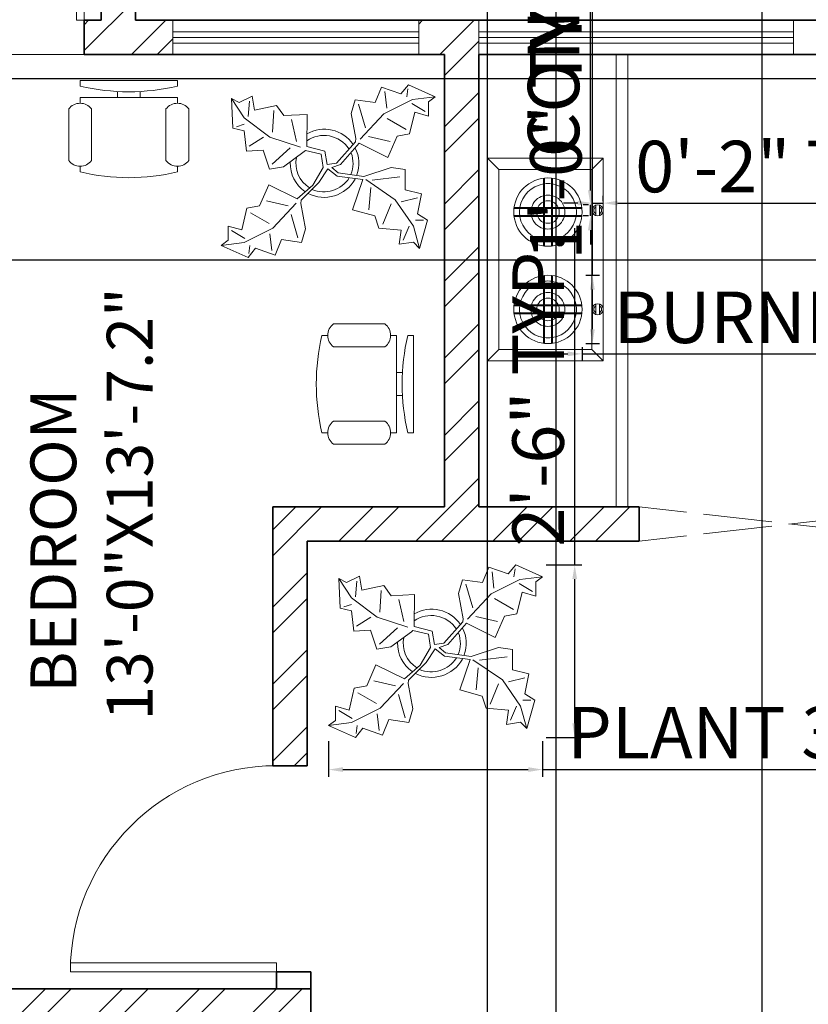
# Model space of a CAD drawing. Units: inches. Extents: x 744 to 1448, y 5126 to 6077.
# Tile 6 of 10: x 895 to 1033, y 5585 to 5757. Entities that reach past the tile are written whole.
import ezdxf

# ---------------------------------------------------------------- set-up
doc = ezdxf.new("R2010")
doc.units = ezdxf.units.IN
doc.linetypes.add('ACAD_ISO02W100', pattern=[15, 12, -3])
for name, color, linetype, lineweight in [('A-ANNO-DIMS', 2, 'Continuous', 18), ('A-AREA-IDEN', 7, 'Continuous', 18), ('A-DOOR', 4, 'Continuous', 18), ('A-EQPM', 9, 'Continuous', 18), ('A-FLOR-CASE', 8, 'Continuous', 18), ('A-FURN', 8, 'Continuous', 18), ('A-WALL', 7, 'Continuous', 35), ('A-WALL-PATT', 252, 'Continuous', 13), ('L-PLNT', 3, 'Continuous', 13)]:
    doc.layers.add(name, color=color, linetype=linetype, lineweight=lineweight)
doc.layers.add('A-GLAZ', color=244, linetype='Continuous', lineweight=18, true_color=0x991b1e)
doc.layers.add('A-WALL-OVHD', color=244, linetype='ACAD_ISO02W100', lineweight=13, true_color=0x991b1e)
doc.styles.get("Standard").update_dxf_attribs({"font": 'arial.ttf'})
doc.dimstyles.new('ISO-25', dxfattribs={"dimtxt": 9, "dimasz": 2.5, "dimexe": 1.25, "dimexo": 0.625, "dimtad": 1, "dimlunit": 3, "dimtxsty": 'Standard', "dimcen": 2.5, "dimadec": 0, "dimazin": 0, "dimtfac": 1, "dimtmove": 0, "dimatfit": 3, "dimfxl": 1, "dimarcsym": 0})

# ---------------------------------------------------------------- blocks, each defined once
blk = doc.blocks.new('*U2')
for p, q in [((0, 0), (0, -6)), ((40, 0), (40, -6))]:
    blk.add_line(p, q)
blk.add_lwpolyline([(0, 0), (0, 40), (1.75, 40), (1.75, 0)], close=True)
blk.add_arc((0, 0), 40, 0, 90)
blk = doc.blocks.new('*U4')
for p, q in [((0, 0), (0, 6)), ((40, 0), (40, 6))]:
    blk.add_line(p, q)
blk.add_lwpolyline([(0, 0), (0, -40), (1.75, -40), (1.75, 0)], close=True)
blk.add_arc((0, 0), 40, 270, 0)
blk = doc.blocks.new('Plant - Rubber or Philodendron')
for p, q in [((13.3837, 12.301), (14.68, 13.9039)), ((14.68, 13.9039), (19.3848, 11.8146)), ((8.8871, 10.7908), (9.9809, 13.4933)), ((9.9809, 13.4933), (13.3837, 12.301)), ((10.5828, 12.6946), (10.8893, 9.7953)), ((14.5816, 13.2037), (14.3848, 11.8033)), ((-16.2005, 11.4774), (-13.9899, 8.1064)), ((-16.2005, 11.4774), (-14.8639, 10.7964)), ((-16.0159, 6.3329), (-16.2005, 11.4774)), ((-14.8639, 10.7964), (-12.6195, 11.8975)), ((-13.3174, 8.325), (-13.0735, 11.0065)), ((-12.6195, 11.8975), (-12.1909, 9.4345)), ((4.6914, 8.8812), (5.3859, 11.2828)), ((5.3859, 11.2828), (8.8871, 10.7908)), ((5.9878, 10.4842), (7.1971, 6.3869)), ((15.3859, 11.3055), (10.3916, 8.7942)), ((15.2875, 10.6053), (17.5907, 9.2105)), ((19.3848, 11.8146), (15.3859, 11.3055)), ((19.3848, 11.8146), (18.1868, 10.9119)), ((18.1868, 10.9119), (18.1925, 8.4119)), ((-12.1909, 9.4345), (-8.3829, 10.3)), ((-8.8369, 9.409), (-9.0894, 5.6095)), ((-8.3829, 10.3), (-7.0549, 8.501)), ((-7.0549, 8.501), (-3.0284, 8.6941)), ((-3.0284, 8.6941), (-3.0709, 3.1041)), ((4.6914, 8.8812), (5.5014, 4.4831)), ((10.3916, 8.7942), (6.2847, 4.4028)), ((15.7909, 9.1065), (14.8995, 5.3044)), ((18.1925, 8.4119), (15.7909, 9.1065)), ((-15.3434, 6.5514), (-13.9984, 6.9884)), ((-13.9899, 8.1064), (-9.5434, 4.7185)), ((-4.8529, 4.012), (-5.7184, 7.82)), ((14.2977, 6.1031), (10.9934, 7.9956)), ((-14.0069, 5.8704), (-16.0159, 6.3329)), ((-13.5868, 2.2894), (-14.0069, 5.8704)), ((14.8995, 5.3044), (12.7005, 4.8994)), ((-13.1329, 3.1804), (-10.6614, 4.727)), ((-9.5434, 4.7185), (-4.1917, 2.9888)), ((2.1141, 0.2298), (5.4346, 3.9146)), ((6.1032, 3.6844), (2.8262, -0.031)), ((5.4346, 3.9146), (5.5014, 4.4831)), ((11.1089, 1.1958), (6.1032, 3.6844)), ((7.7005, 4.8881), (11.5025, 3.9967)), ((12.7005, 4.8994), (11.1089, 1.1958)), ((-10.6784, 2.491), (-13.5868, 2.2894)), ((-9.5858, -0.8715), (-10.6784, 2.491)), ((-9.1318, 0.0195), (-5.9793, 2.9025)), ((-7.1228, -0.443), (-3.5248, 2.2131)), ((-3.5248, 2.2131), (-3.3011, 2.4355)), ((-3.3011, 2.4355), (-0.5306, 1.7947)), ((-3.0709, 3.1041), (0.0797, 2.3163)), ((-0.5306, 1.7947), (-0.2255, -0.5527)), ((-0.5306, 1.7947), (-0.5306, 1.7947)), ((0.0797, 2.3163), (0.4866, -0.031)), ((0.4866, -0.031), (2.1141, 0.2298)), ((-7.1228, -0.443), (-9.5858, -0.8715)), ((-2.019, -3.6148), (-0.2255, -0.5527)), ((-0.9375, -3.1608), (0.5883, -0.8135)), ((0.5883, -0.8135), (2.2447, -2.0916)), ((2.8262, -0.031), (1.3003, -0.5527)), ((1.3003, -0.5527), (2.4193, -1.4655)), ((2.4193, -1.4655), (6.895, -2.1175)), ((11.6605, -0.5413), (6.895, -2.1175)), ((11.6605, -0.5413), (14.1354, -0.8948)), ((14.1354, -0.8948), (14.1354, -4.4304)), ((-4.0579, -6.2781), (-0.9375, -3.1608)), ((2.2447, -2.0916), (6.7108, -2.6626)), ((4.943, -7.9659), (6.7108, -2.6626)), ((12.3677, -6.1981), (7.219, -2.6772)), ((8.3544, -2.7453), (13.1973, -2.1704)), ((-11.3237, -7.2629), (-9.7321, -3.5593)), ((-9.7321, -3.5593), (-4.7264, -6.0479)), ((-2.019, -3.6148), (-4.7264, -6.0479)), ((8.125, -4.0768), (7.7715, -7.9659)), ((14.1354, -4.4304), (16.9638, -5.1375)), ((16.9638, -5.1375), (16.2567, -8.673)), ((-6.3237, -7.2516), (-10.1257, -6.3602)), ((-9.0148, -11.1577), (-4.9047, -6.8122)), ((-4.1246, -6.8466), (-4.0579, -6.2781)), ((-3.3146, -11.2447), (-4.1246, -6.8466)), ((15.5496, -10.7943), (12.3677, -6.1981)), ((16.2567, -5.8446), (13.4283, -6.5517)), ((-14.4141, -11.4699), (-13.5228, -7.6679)), ((-13.5228, -7.6679), (-11.3237, -7.2629)), ((-12.921, -8.4665), (-9.6166, -10.359)), ((8.8321, -9.0266), (4.943, -7.9659)), ((10.2463, -10.4408), (11.6605, -6.9053)), ((-4.611, -12.8477), (-5.8203, -8.7504)), ((9.5392, -11.1479), (8.8321, -9.0266)), ((17.3174, -9.7337), (15.9032, -9.7337)), ((16.2567, -8.673), (18.0245, -9.7337)), ((18.0245, -9.7337), (16.6103, -14.6834)), ((-16.8157, -10.7754), (-14.4141, -11.4699)), ((-16.8101, -13.2754), (-16.8157, -10.7754)), ((-13.9107, -12.9688), (-16.2139, -11.574)), ((-14.0091, -13.669), (-9.0148, -11.1577)), ((-3.3146, -11.2447), (-4.0092, -13.6463)), ((13.4283, -11.5015), (9.5392, -11.1479)), ((13.0748, -13.9763), (13.4283, -11.5015)), ((14.8425, -10.7943), (13.7819, -13.2692)), ((16.6103, -14.6834), (15.5496, -10.7943)), ((-18.008, -14.1781), (-16.8101, -13.2754)), ((-18.008, -14.1781), (-14.0091, -13.669)), ((-9.206, -15.0581), (-9.5126, -12.1588)), ((-7.5103, -13.1543), (-8.6042, -15.8568)), ((-4.0092, -13.6463), (-7.5103, -13.1543)), ((15.5496, -13.6228), (13.0748, -13.9763)), ((16.6103, -14.6834), (15.5496, -13.6228)), ((-13.3032, -16.2674), (-18.008, -14.1781)), ((-12.0069, -14.6645), (-13.3032, -16.2674)), ((-13.2048, -15.5672), (-13.008, -14.1668)), ((-8.6042, -15.8568), (-12.0069, -14.6645))]:
    blk.add_line(p, q)
for centre, radius, start, end in [((0, 0), 6.1275, 34.37569, 120.1028), ((-0.0601, -0.2075), 5.2461, 33.82192, 124.9414), ((-0.2664, 0.1682), 5.2775, 338.4094, 20.03007), ((-0.098, 0.1364), 6.1288, 341.2017, 26.09184), ((0.0308, 0.1664), 6, 178.6147, 235.1169), ((0.0308, 0.1664), 5, 168.1647, 238.6725), ((-0.0234, 0.3825), 6.1492, 242.5812, 331.2714), ((-0.1102, 0.4886), 5.2883, 247.3711, 327.472)]:
    blk.add_arc(centre, radius, start, end)
blk = doc.blocks.new('Chair - Desk')
for p, q in [((-8.5, 0), (-8.5, -1)), ((-8.5, 0), (8.5, 0)), ((8.5, 0), (8.5, -1)), ((-8.5, -3), (-8.5, -4)), ((-8.5, -3), (8.5, -3)), ((-2, -3), (-2, -1.9355)), ((2, -1.9576), (2, -3)), ((8.5, -3), (8.5, -4)), ((-10.5, -5), (-10.5, -14)), ((-6.5, -14), (-6.5, -5)), ((6.5, -5), (6.5, -14)), ((10.5, -14), (10.5, -5)), ((-8.5, -15), (-8.5, -16)), ((8.5, -15), (8.5, -16))]:
    blk.add_line(p, q)
for centre, radius, start, end in [((0, 34.625), 36.625, 256.5803, 283.4197), ((-8.5, -6.5), 2.5, 36.8699, 143.1301), ((8.5, -6.5), 2.5, 36.8699, 143.1301), ((-8.5, -12.5), 2.5, 216.8699, 323.1301), ((8.5, -12.5), 2.5, 216.8699, 323.1301), ((0, 19.625), 36.625, 256.5803, 283.4197)]:
    blk.add_arc(centre, radius, start, end)
blk = doc.blocks.new('WINDOW-GLASS-55IN')
for p, q in [((0, 2), (55, 2)), ((0, 1), (55, 1)), ((0, 0), (55, 0))]:
    blk.add_line(p, q)
blk = doc.blocks.new('WINDOW-GLASS-43IN')
for p, q in [((0, 2), (43, 2)), ((0, 1), (43, 1)), ((0, 0), (43, 0))]:
    blk.add_line(p, q)
blk = doc.blocks.new('COOKTOP-BURNER')
for p, q in [((5.17, 0.05), (5.17, 11.89)), ((5.37, 6.77), (5.37, 11.91)), ((6.57, 6.77), (6.57, 11.91)), ((6.77, 0.05), (6.77, 11.89)), ((0.03, 6.57), (5.17, 6.57)), ((0.03, 5.37), (5.17, 5.37)), ((0.05, 6.77), (11.89, 6.77)), ((0.05, 5.17), (11.89, 5.17)), ((5.37, 6.57), (6.57, 6.57)), ((5.37, 5.37), (5.37, 6.57)), ((5.37, 5.37), (6.57, 5.37)), ((5.37, 0.03), (5.37, 5.17)), ((6.57, 5.37), (6.57, 6.57)), ((6.57, 0.03), (6.57, 5.17)), ((6.77, 6.57), (11.91, 6.57)), ((6.77, 5.37), (11.91, 5.37))]:
    blk.add_line(p, q)
blk.add_circle((5.97, 5.97), 5.97)
for radius, start, end in [(4.97, 99.2606, 170.7394), (4.97, 83.0678, 96.9322), (4.97, 9.2606, 80.7394), (2.97, 105.6195, 164.3805), (2.97, 78.3498, 101.6502), (2.97, 15.6195, 74.3805), (1.97, 113.9436, 156.0564), (1.97, 72.2793, 107.7207), (1.97, 23.9436, 66.0564), (4.97, 173.0678, 186.9322), (4.97, 189.2606, 260.7394), (2.97, 168.3498, 191.6502), (2.97, 195.6195, 254.3805), (1.97, 162.2793, 197.7207), (1.97, 203.9436, 246.0564), (4.97, 279.2606, 350.7394), (2.97, 285.6195, 344.3805), (1.97, 293.9436, 336.0564), (1.97, 342.2793, 17.7207), (2.97, 348.3498, 11.6502), (4.97, 353.0678, 6.9322), (1.97, 252.2793, 287.7207), (2.97, 258.3498, 281.6502), (4.97, 263.0678, 276.9322)]:
    blk.add_arc((5.97, 5.97), radius, start, end)
blk = doc.blocks.new('COOKTOP-CONTROL')
for p, q in [((0.68, 1.91), (0.68, 0.05)), ((1.28, 1.91), (1.28, 0.05))]:
    blk.add_line(p, q)
blk.add_circle((0.98, 0.98), 0.979)
for start, end in [(116.2244, 243.7756), (296.2244, 63.7756)]:
    blk.add_arc((0.98, 0.98), 0.679, start, end)
blk = doc.blocks.new('*D35')
at = {"layer": 'A-ANNO-DIMS', "color": 0, "lineweight": -2, "transparency": 16777216}
for p, q in [((949.42, 5630.92), (949.42, 5624.68)), ((986.81, 5630.92), (986.81, 5624.68)), ((951.92, 5625.93), (984.31, 5625.93)), ((986.81, 5625.93), (1109.97, 5625.93))]:
    blk.add_line(p, q, dxfattribs=at)
at = {"layer": 'A-ANNO-DIMS', "color": 0, "transparency": 16777216}
for points in [[(951.92, 5626.35), (951.92, 5625.52), (949.42, 5625.93)], [(984.31, 5626.35), (984.31, 5625.52), (986.81, 5625.93)]]:
    blk.add_solid(points, dxfattribs=at)
at = {"layer": 'Defpoints', "color": 0, "transparency": 16777216}
for p in [(949.42, 5631.54), (986.81, 5631.54), (986.81, 5625.93)]:
    blk.add_point(p, dxfattribs=at)
at = {"layer": 'A-ANNO-DIMS', "color": 0, "transparency": 16777216, "insert": (1049.64, 5631.22), "char_height": 9, "attachment_point": 5}
blk.add_mtext('PLANT 3\'-1 1/2" TYP.', dxfattribs=at)
blk = doc.blocks.new('*D36')
at = {"layer": 'A-ANNO-DIMS', "color": 0, "lineweight": -2, "transparency": 16777216}
for p, q in [((992.42, 5661.71), (992.42, 5720.48)), ((987.44, 5661.71), (993.67, 5661.71)), ((992.42, 5634.04), (992.42, 5659.21)), ((987.44, 5631.54), (993.67, 5631.54))]:
    blk.add_line(p, q, dxfattribs=at)
at = {"layer": 'A-ANNO-DIMS', "color": 0, "transparency": 16777216}
for points in [[(992.01, 5659.21), (992.84, 5659.21), (992.42, 5661.71)], [(992.01, 5634.04), (992.84, 5634.04), (992.42, 5631.54)]]:
    blk.add_solid(points, dxfattribs=at)
at = {"layer": 'Defpoints', "color": 0, "transparency": 16777216}
for p in [(986.81, 5661.71), (992.42, 5661.71), (986.81, 5631.54)]:
    blk.add_point(p, dxfattribs=at)
at = {"layer": 'A-ANNO-DIMS', "color": 0, "transparency": 16777216, "insert": (987.2, 5692.35), "char_height": 9, "attachment_point": 5, "rotation": 90}
blk.add_mtext('2\'-6" TYP.', dxfattribs=at)
blk = doc.blocks.new('*D49')
at = {"layer": 'A-ANNO-DIMS', "color": 0, "lineweight": -2, "transparency": 16777216}
for p, q in [((981.78, 5699.72), (981.78, 5697.3)), ((984.28, 5698.55), (991.22, 5698.55)), ((993.72, 5699.72), (993.72, 5697.3)), ((993.72, 5698.55), (1108.52, 5698.55))]:
    blk.add_line(p, q, dxfattribs=at)
at = {"layer": 'A-ANNO-DIMS', "color": 0, "transparency": 16777216}
for points in [[(984.28, 5698.97), (984.28, 5698.14), (981.78, 5698.55)], [(991.22, 5698.97), (991.22, 5698.14), (993.72, 5698.55)]]:
    blk.add_solid(points, dxfattribs=at)
at = {"layer": 'Defpoints', "color": 0, "transparency": 16777216}
for p in [(981.78, 5700.35), (993.72, 5700.35), (993.72, 5698.55)]:
    blk.add_point(p, dxfattribs=at)
at = {"layer": 'A-ANNO-DIMS', "color": 0, "transparency": 16777216, "insert": (1052.37, 5703.77), "char_height": 9, "attachment_point": 5}
blk.add_mtext('BURNER 1\'-0" TYP.', dxfattribs=at)
blk = doc.blocks.new('*D50')
at = {"layer": 'A-ANNO-DIMS', "color": 0, "lineweight": -2, "transparency": 16777216}
for p, q in [((995.52, 5712.29), (995.52, 5770.05)), ((994.35, 5712.29), (996.77, 5712.29)), ((995.52, 5702.85), (995.52, 5709.79)), ((994.35, 5700.35), (996.77, 5700.35))]:
    blk.add_line(p, q, dxfattribs=at)
at = {"layer": 'A-ANNO-DIMS', "color": 0, "transparency": 16777216}
for points in [[(995.1, 5709.79), (995.93, 5709.79), (995.52, 5712.29)], [(995.1, 5702.85), (995.93, 5702.85), (995.52, 5700.35)]]:
    blk.add_solid(points, dxfattribs=at)
at = {"layer": 'Defpoints', "color": 0, "transparency": 16777216}
for p in [(993.72, 5712.29), (995.52, 5712.29), (993.72, 5700.35)]:
    blk.add_point(p, dxfattribs=at)
at = {"layer": 'A-ANNO-DIMS', "color": 0, "transparency": 16777216, "insert": (990.3, 5742.42), "char_height": 9, "attachment_point": 5, "rotation": 90}
blk.add_mtext('1\'-0" TYP.', dxfattribs=at)
blk = doc.blocks.new('*D51')
at = {"layer": 'A-ANNO-DIMS', "color": 0, "lineweight": -2, "transparency": 16777216}
for p, q in [((995.17, 5727.09), (995.17, 5850.56)), ((994.84, 5724.59), (993.92, 5724.59)), ((995.17, 5722.64), (995.17, 5724.59)), ((994.84, 5722.64), (993.92, 5722.64)), ((995.17, 5720.14), (995.17, 5717.64))]:
    blk.add_line(p, q, dxfattribs=at)
at = {"layer": 'A-ANNO-DIMS', "color": 0, "transparency": 16777216}
for points in [[(994.75, 5727.09), (995.58, 5727.09), (995.17, 5724.59)], [(994.75, 5720.14), (995.58, 5720.14), (995.17, 5722.64)]]:
    blk.add_solid(points, dxfattribs=at)
at = {"layer": 'Defpoints', "color": 0, "transparency": 16777216}
for p in [(995.17, 5724.59), (995.46, 5724.59), (995.46, 5722.64)]:
    blk.add_point(p, dxfattribs=at)
at = {"layer": 'A-ANNO-DIMS', "color": 0, "transparency": 16777216, "insert": (989.89, 5790.08), "char_height": 9, "attachment_point": 5, "rotation": 90}
blk.add_mtext('CONTROL 0\'-2" TYP.', dxfattribs=at)
blk = doc.blocks.new('*D52')
at = {"layer": 'A-ANNO-DIMS', "color": 0, "lineweight": -2, "transparency": 16777216}
for p, q in [((995.46, 5725.22), (995.46, 5726.14)), ((997.42, 5725.22), (997.42, 5726.14)), ((992.96, 5724.89), (990.46, 5724.89)), ((995.46, 5724.89), (997.42, 5724.89)), ((999.92, 5724.89), (1058.53, 5724.89))]:
    blk.add_line(p, q, dxfattribs=at)
at = {"layer": 'A-ANNO-DIMS', "color": 0, "transparency": 16777216}
for points in [[(992.96, 5725.3), (992.96, 5724.47), (995.46, 5724.89)], [(999.92, 5725.3), (999.92, 5724.47), (997.42, 5724.89)]]:
    blk.add_solid(points, dxfattribs=at)
at = {"layer": 'Defpoints', "color": 0, "transparency": 16777216}
for p in [(995.46, 5724.59), (997.42, 5724.89), (997.42, 5724.59)]:
    blk.add_point(p, dxfattribs=at)
at = {"layer": 'A-ANNO-DIMS', "color": 0, "transparency": 16777216, "insert": (1030.47, 5730.11), "char_height": 9, "attachment_point": 5}
blk.add_mtext('0\'-2" TYP.', dxfattribs=at)
blk = doc.blocks.new('*D55')
at = {"layer": 'A-ANNO-DIMS', "color": 0, "lineweight": -2, "transparency": 16777216}
for p, q in [((989.18, 5323.94), (989.18, 6059.61)), ((1025.18, 5323.94), (1025.18, 6059.61)), ((991.68, 6058.36), (1022.68, 6058.36))]:
    blk.add_line(p, q, dxfattribs=at)
at = {"layer": 'A-ANNO-DIMS', "color": 0, "transparency": 16777216}
for points in [[(991.68, 6058.78), (991.68, 6057.95), (989.18, 6058.36)], [(1022.68, 6058.78), (1022.68, 6057.95), (1025.18, 6058.36)]]:
    blk.add_solid(points, dxfattribs=at)
at = {"layer": 'Defpoints', "color": 0, "transparency": 16777216}
for p in [(1025.18, 6058.36), (989.18, 5323.32), (1025.18, 5323.32)]:
    blk.add_point(p, dxfattribs=at)
at = {"layer": 'A-ANNO-DIMS', "color": 0, "transparency": 16777216, "insert": (1007.18, 6063.59), "char_height": 9, "attachment_point": 5}
blk.add_mtext('3\'-0"', dxfattribs=at)
blk = doc.blocks.new('*D59')
at = {"layer": 'A-ANNO-DIMS', "color": 0, "lineweight": -2, "transparency": 16777216}
for p, q in [((762.28, 5746.58), (762.28, 5795.38)), ((1128.24, 5746.58), (761.03, 5746.58)), ((762.28, 5717.4), (762.28, 5744.08)), ((1128.24, 5714.9), (761.03, 5714.9))]:
    blk.add_line(p, q, dxfattribs=at)
at = {"layer": 'A-ANNO-DIMS', "color": 0, "transparency": 16777216}
for points in [[(761.87, 5744.08), (762.7, 5744.08), (762.28, 5746.58)], [(761.87, 5717.4), (762.7, 5717.4), (762.28, 5714.9)]]:
    blk.add_solid(points, dxfattribs=at)
at = {"layer": 'Defpoints', "color": 0, "transparency": 16777216}
for p in [(762.28, 5746.58), (1128.86, 5746.58), (1128.86, 5714.9)]:
    blk.add_point(p, dxfattribs=at)
at = {"layer": 'A-ANNO-DIMS', "color": 0, "transparency": 16777216, "insert": (757.01, 5772.23), "char_height": 9, "attachment_point": 5, "rotation": 90}
blk.add_mtext('2\'-7 1/2"', dxfattribs=at)
blk = doc.blocks.new('*D62')
at = {"layer": 'A-ANNO-DIMS', "color": 0, "lineweight": -2, "transparency": 16777216}
for p, q in [((816.68, 5262.94), (816.68, 6059.61)), ((977.18, 5262.94), (977.18, 6059.61)), ((819.18, 6058.36), (974.68, 6058.36))]:
    blk.add_line(p, q, dxfattribs=at)
at = {"layer": 'A-ANNO-DIMS', "color": 0, "transparency": 16777216}
for points in [[(819.18, 6058.78), (819.18, 6057.95), (816.68, 6058.36)], [(974.68, 6058.78), (974.68, 6057.95), (977.18, 6058.36)]]:
    blk.add_solid(points, dxfattribs=at)
at = {"layer": 'Defpoints', "color": 0, "transparency": 16777216}
for p in [(977.18, 6058.36), (816.68, 5262.32), (977.18, 5262.32)]:
    blk.add_point(p, dxfattribs=at)
at = {"layer": 'A-ANNO-DIMS', "color": 0, "transparency": 16777216, "insert": (896.93, 6063.64), "char_height": 9, "attachment_point": 5}
blk.add_mtext('13\'-4 1/2"', dxfattribs=at)

msp = doc.modelspace()

# ---------------------------------------------------------------- hatches: boundary and pattern name
at = {"layer": 'A-WALL-PATT'}
h = msp.add_hatch(dxfattribs=at)
h.set_pattern_fill('ANSI32', color=256)
h.paths.add_polyline_path([(813.684, 5750.816), (876.684, 5750.816), (876.684, 5756.816), (813.684, 5756.816), (813.684, 5812.816), (909.684, 5812.816), (909.684, 5795.316), (915.684, 5795.316), (915.684, 5812.816), (1209.684, 5812.816), (1209.684, 5795.316), (1215.684, 5795.316), (1215.684, 5812.816), (1311.684, 5812.816), (1311.684, 5756.816), (1248.684, 5756.816), (1248.684, 5750.816), (1311.684, 5750.816), (1311.684, 5570.816), (1179.044, 5570.816), (1179.044, 5564.816), (1311.684, 5564.816), (1311.684, 5383.316), (1260.684, 5383.316), (1260.684, 5377.316), (1311.684, 5377.316), (1311.684, 5320.316), (1227.684, 5320.316), (1227.684, 5333.816), (1221.684, 5333.816), (1221.684, 5314.316), (1320.684, 5314.316), (1320.684, 5821.816), (804.684, 5821.816), (804.684, 5472.316), (926.184, 5472.316), (926.184, 5481.316), (813.684, 5481.316), (813.684, 5581.616), (946.284, 5581.616), (946.284, 5587.616), (813.684, 5587.616)])
h.paths.add_polyline_path([(1155.684, 5525.816), (1149.684, 5525.816), (1149.684, 5481.316), (1025.184, 5481.316), (1025.184, 5475.316), (1146.684, 5475.316), (1146.684, 5323.316), (1118.788, 5323.316), (1118.788, 5314.316), (1146.684, 5314.316), (1155.684, 5314.316), (1155.684, 5374.316), (1170.35, 5374.316), (1170.35, 5383.316), (1155.684, 5383.316)], flags=17)
h.paths.add_polyline_path([(1230.684, 5383.316), (1213.35, 5383.316), (1213.35, 5374.316), (1221.684, 5374.316), (1221.684, 5363.816), (1226.184, 5363.816), (1227.684, 5363.816), (1227.684, 5377.316), (1230.684, 5377.316)], flags=17)
h.paths.add_polyline_path([(1185.684, 5671.816), (1155.684, 5671.816), (1155.684, 5750.816), (1161.575, 5750.816), (1161.575, 5756.816), (1157.542, 5756.816), (1157.847, 5756.715), (1155.79, 5756.816), (1149.684, 5756.816), (1149.684, 5750.816), (1149.684, 5671.816), (1121.684, 5671.816), (1121.684, 5665.816), (1179.684, 5665.816), (1179.684, 5609.816), (1185.684, 5609.816)], flags=17)
h.paths.add_polyline_path([(1003.684, 5671.816), (975.684, 5671.816), (975.684, 5750.816), (975.684, 5756.816), (965.205, 5756.816), (965.205, 5750.816), (969.684, 5750.816), (969.684, 5671.816), (939.684, 5671.816), (939.684, 5626.616), (945.684, 5626.616), (945.684, 5665.816), (1003.684, 5665.816)], flags=17)
h.paths.add_polyline_path([(915.684, 5774.316), (909.684, 5774.316), (909.684, 5756.816), (906.684, 5756.816), (906.684, 5752.316), (906.684, 5750.816), (922.205, 5750.816), (922.205, 5756.816), (915.684, 5756.816)], flags=17)
h.paths.add_polyline_path([(1215.684, 5774.316), (1209.684, 5774.316), (1209.684, 5756.816), (1204.575, 5756.816), (1204.575, 5750.816), (1218.684, 5750.816), (1218.684, 5756.816), (1215.684, 5756.816)], flags=17)
h.paths.add_polyline_path([(1063.788, 5323.316), (1025.184, 5323.316), (1025.184, 5314.316), (1063.788, 5314.316)])
h.paths.add_polyline_path([(986.184, 5475.316), (989.184, 5475.316), (989.184, 5481.316), (974.184, 5481.316), (974.184, 5475.916), (974.184, 5472.316), (977.184, 5472.316), (977.184, 5314.316), (989.184, 5314.316), (989.184, 5319.716), (989.184, 5323.316), (986.184, 5323.316)])

# ---------------------------------------------------------------- linework, layer by layer
at = {"layer": 'A-DOOR'}
msp.add_line((876.684, 5750.816), (906.684, 5750.816), dxfattribs=at)
at = {"layer": 'A-EQPM'}
for p, q in [((979.168, 5730.754), (977.168, 5732.754)), ((995.402, 5730.754), (997.402, 5732.754)), ((979.168, 5699.336), (977.168, 5697.336)), ((995.402, 5699.336), (997.402, 5697.336))]:
    msp.add_line(p, q, dxfattribs=at)
for points in [[(977.168, 5732.754), (997.402, 5732.754), (997.402, 5697.336), (977.168, 5697.336)], [(979.168, 5730.754), (995.402, 5730.754), (995.402, 5699.336), (979.168, 5699.336)]]:
    msp.add_lwpolyline(points, close=True, dxfattribs=at)
at = {"layer": 'A-FLOR-CASE'}
for p, q in [((999.684, 5671.816), (999.684, 5750.816)), ((1001.684, 5671.816), (1001.684, 5750.816))]:
    msp.add_line(p, q, dxfattribs=at)
at = {"layer": 'A-GLAZ'}
for points in [[(922.205, 5756.816), (965.205, 5756.816), (965.205, 5750.816), (922.205, 5750.816)], [(975.684, 5756.816), (1030.684, 5756.816), (1030.684, 5750.816), (975.684, 5750.816)]]:
    msp.add_lwpolyline(points, close=True, dxfattribs=at)
at = {"layer": 'A-WALL'}
for p, q in [((909.684, 5756.816), (909.684, 5812.816)), ((915.684, 5756.816), (915.684, 5812.816)), ((906.684, 5756.816), (906.684, 5750.816)), ((906.684, 5756.816), (909.684, 5756.816)), ((915.684, 5756.816), (1038.684, 5756.816)), ((906.684, 5750.816), (969.684, 5750.816)), ((969.684, 5671.816), (969.684, 5750.816)), ((975.684, 5750.816), (1038.684, 5750.816)), ((975.684, 5671.816), (975.684, 5750.816)), ((939.684, 5671.816), (969.684, 5671.816)), ((939.684, 5626.616), (939.684, 5671.816)), ((975.684, 5671.816), (1003.684, 5671.816)), ((1003.684, 5665.816), (1003.684, 5671.816)), ((945.684, 5665.816), (1003.684, 5665.816)), ((945.684, 5626.616), (945.684, 5665.816)), ((945.684, 5626.616), (939.684, 5626.616)), ((940.284, 5587.616), (940.284, 5590.616)), ((940.284, 5590.616), (946.284, 5590.616)), ((946.284, 5590.616), (946.284, 5581.616)), ((813.684, 5587.616), (946.284, 5587.616))]:
    msp.add_line(p, q, dxfattribs=at)
at = {"layer": 'A-WALL-OVHD'}
for p, q in [((1056.684, 5665.816), (1003.684, 5671.816)), ((1056.684, 5671.816), (1003.684, 5665.816))]:
    msp.add_line(p, q, dxfattribs=at)

# ---------------------------------------------------------------- block references
at = {"layer": 'A-DOOR'}
for name, p, xscale, yscale, zscale, rotation in [('*U4', (906.684, 5756.816), 0.75, 0.75, 0.75, 180.0000000000004), ('*U2', (940.284, 5590.616), 0.9, 0.9, 0.9, 90)]:
    msp.add_blockref(name, p, dxfattribs=dict(at, xscale=xscale, yscale=yscale, zscale=zscale, rotation=rotation))
at = {"layer": 'A-EQPM'}
for name, p, rotation in [('COOKTOP-BURNER', (993.724, 5717.353), 90.00000000001334), ('COOKTOP-CONTROL', (997.419, 5707.321), 180)]:
    msp.add_blockref(name, p, dxfattribs=dict(at, rotation=rotation))
for name, p in [('COOKTOP-CONTROL', (995.462, 5722.636)), ('COOKTOP-BURNER', (981.782, 5700.346))]:
    msp.add_blockref(name, p, dxfattribs=at)
at = {"layer": 'A-FURN'}
msp.add_blockref('Chair - Desk', (914.494, 5746.329), dxfattribs=at)
at = {"layer": 'A-FURN', "rotation": 270}
msp.add_blockref('Chair - Desk', (964.261, 5693.281), dxfattribs=at)
at = {"layer": 'A-GLAZ'}
for name, p in [('WINDOW-GLASS-43IN', (922.205, 5752.816)), ('WINDOW-GLASS-55IN', (975.684, 5752.816))]:
    msp.add_blockref(name, p, dxfattribs=at)
at = {"layer": 'L-PLNT'}
for p in [(948.674, 5731.662), (967.43, 5647.811)]:
    msp.add_blockref('Plant - Rubber or Philodendron', p, dxfattribs=at)

# ---------------------------------------------------------------- texts
at = {"layer": 'A-AREA-IDEN', "insert": (897.314, 5634.491), "char_height": 8, "attachment_point": 1, "rotation": 90}
msp.add_mtext_dynamic_manual_height_columns('  BEDROOM\\P13\'-0"X13\'-7.2"', width=74.03424, gutter_width=12.5, heights=[0], dxfattribs=at)

# ---------------------------------------------------------------- dimensions: what is measured, and where the dimension line sits
at = {"layer": 'A-ANNO-DIMS'}
for base, p1, p2, picture, middle in [((977.184, 6058.363), (816.684, 5262.316), (977.184, 5262.316), '*D62', (896.934, 6063.645)), ((1025.184, 6058.363), (989.184, 5323.316), (1025.184, 5323.316), '*D55', (1007.184, 6063.586))]:
    dim = msp.add_linear_dim(base=base, p1=p1, p2=p2, dimstyle='ISO-25', override={"dimdec": 1, "dimlfac": 1, "dimrnd": 0, "dimzin": 1, "dimdsep": 46, "dimlunit": 4, "dimfrac": 2}, dxfattribs=at)
    dim.commit()
    dim.dimension.update_dxf_attribs({"geometry": picture, "text_midpoint": middle})
for base, p1, p2, text, picture, middle in [((995.168, 5724.594), (995.462, 5722.636), (995.462, 5724.594), 'CONTROL <> TYP.', '*D51', (989.886, 5790.079)), ((995.516, 5712.288), (993.724, 5700.346), (993.724, 5712.288), '<> TYP.', '*D50', (990.296, 5742.42)), ((992.424, 5661.715), (986.815, 5631.544), (986.815, 5661.715), '<> TYP.', '*D36', (987.204, 5692.346))]:
    dim = msp.add_linear_dim(base=base, p1=p1, p2=p2, angle=90, text=text, dimstyle='ISO-25', override={"dimdec": 1, "dimlfac": 1, "dimrnd": 0, "dimzin": 1, "dimdsep": 46, "dimlunit": 4, "dimfrac": 2}, dxfattribs=at)
    dim.commit()
    dim.dimension.update_dxf_attribs({"geometry": picture, "text_midpoint": middle})
dim = msp.add_linear_dim(base=(762.284, 5746.584), p1=(1128.864, 5714.896), p2=(1128.864, 5746.584), angle=90, dimstyle='ISO-25', override={"dimdec": 1, "dimlfac": 1, "dimrnd": 0, "dimzin": 1, "dimdsep": 46, "dimlunit": 4, "dimfrac": 2}, dxfattribs=at)
dim.commit()
dim.dimension.update_dxf_attribs({"geometry": '*D59', "text_midpoint": (757.006, 5772.234)})
for base, p1, p2, text, picture, middle in [((997.419, 5724.887), (995.462, 5724.594), (997.419, 5724.594), '<> TYP.', '*D52', (1030.474, 5730.108)), ((993.724, 5698.555), (981.782, 5700.346), (993.724, 5700.346), 'BURNER <> TYP.', '*D49', (1052.372, 5703.775)), ((986.815, 5625.935), (949.422, 5631.544), (986.815, 5631.544), 'PLANT <> TYP.', '*D35', (1049.64, 5631.216))]:
    dim = msp.add_linear_dim(base=base, p1=p1, p2=p2, text=text, dimstyle='ISO-25', override={"dimdec": 1, "dimlfac": 1, "dimrnd": 0, "dimzin": 1, "dimdsep": 46, "dimlunit": 4, "dimfrac": 2}, dxfattribs=at)
    dim.commit()
    dim.dimension.update_dxf_attribs({"geometry": picture, "text_midpoint": middle})

doc.saveas('drawing.dxf')
